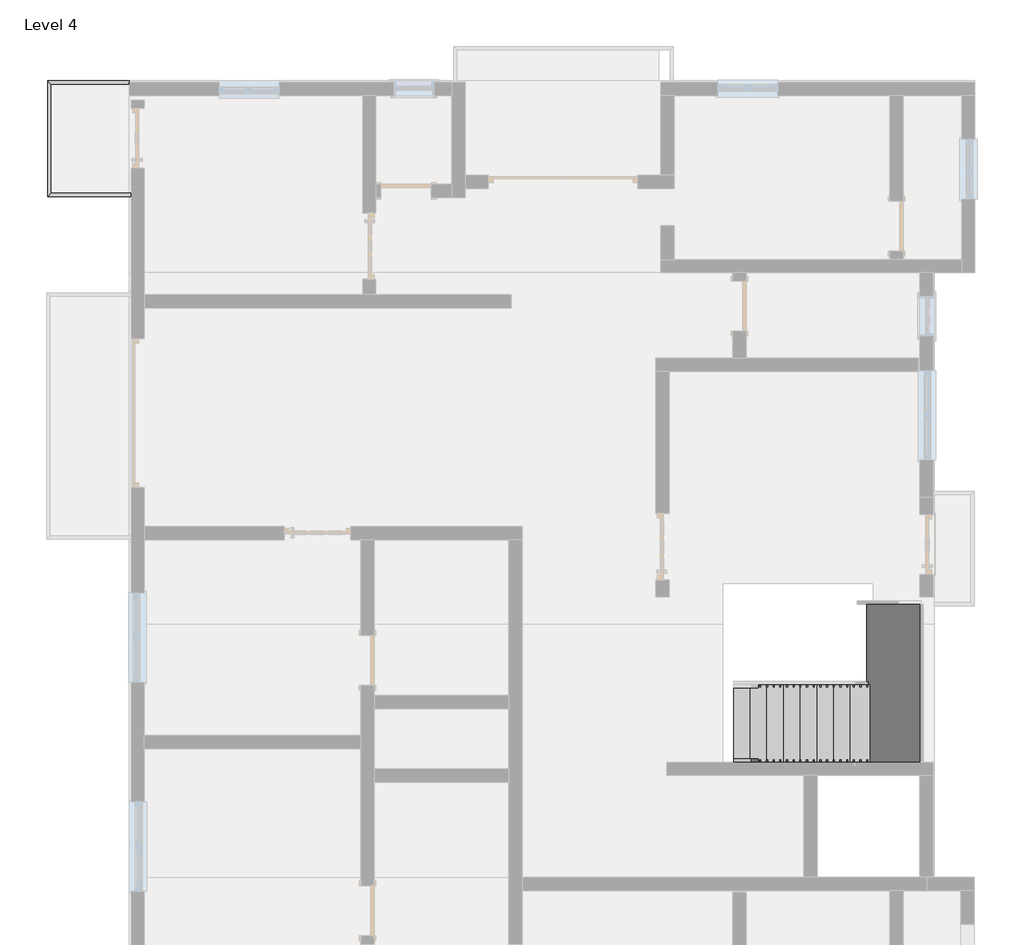
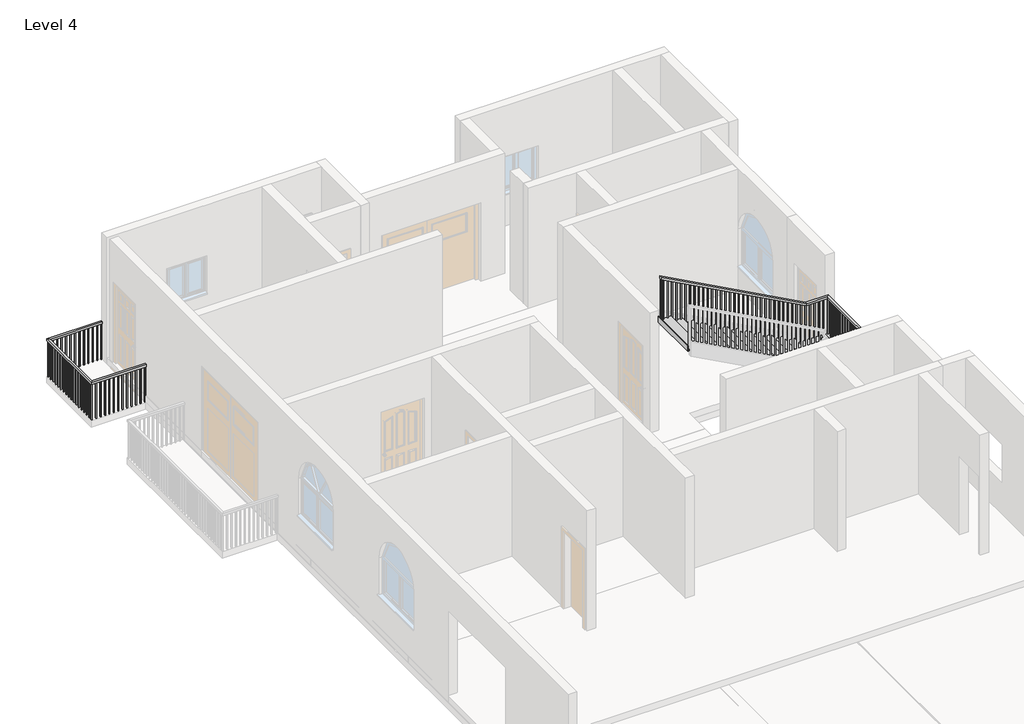
# One storey, part 5 of 7: 2 railings, 1 stair flight.
"""IFC4 building model written with IfcOpenShell, lengths in millimetres."""

from ifc_helpers import new_model, si_unit, frame, origin, place, context, project, spatial, polyline, outline, extrude, faceted_brep, transform, mapped, element, save
from components import stair_flight_9b376cb7

model = new_model("IFC4")

# Units and contexts
model_context = context("Model", 3, world=origin())
ifc_project = project(units=[si_unit("LENGTHUNIT", "METRE", prefix="MILLI")], contexts=[model_context])

# Site, building, storey
site = spatial("IfcSite", under=ifc_project)
building = spatial("IfcBuilding", under=site)
storey = spatial("IfcBuildingStorey", under=building, Name="Level 4", Elevation=9144.0)

# Railings
placement = place(None, origin())
element("IfcRailing", 1, ObjectType="Handrail - Rectangular", at=placement, inside=storey, context=model_context, shape_type="SolidModel", body=[
    faceted_brep([(-6354.2109037, 9376.4527313, 10058.4), (-6354.2109037, 9376.4527313, 10007.6), (-6354.2109037, 9427.2527313, 10007.6), (-6354.2109037, 9427.2527313, 10058.4), (-7548.0109037, 9376.4527313, 10058.4), (-7548.0109037, 9376.4527313, 10007.6), (-7598.8109037, 9427.2527313, 10007.6), (-7598.8109037, 9427.2527313, 10058.4), (-7548.0109037, 7717.9584215, 10058.4), (-7548.0109037, 7717.9584215, 10007.6), (-7598.8109037, 7667.1584215, 10007.6), (-7598.8109037, 7667.1584215, 10058.4), (-6330.8013636, 7717.9584215, 10058.4), (-6330.8013636, 7667.1584215, 10058.4), (-6330.8013636, 7667.1584215, 10007.6), (-6330.8013636, 7717.9584215, 10007.6)], [[[0, 1, 2, 3]], [[1, 0, 4, 5]], [[2, 1, 5, 6]], [[3, 2, 6, 7]], [[0, 3, 7, 4]], [[5, 4, 8, 9]], [[6, 5, 9, 10]], [[7, 6, 10, 11]], [[4, 7, 11, 8]], [[12, 13, 14, 15]], [[9, 8, 12, 15]], [[10, 9, 15, 14]], [[11, 10, 14, 13]], [[8, 11, 13, 12]]]),
    extrude(outline(polyline([(-6363.7359037, 7683.0334215), (-6363.7359037, 7702.0834215), (-6344.6859037, 7702.0834215), (-6344.6859037, 7683.0334215), (-6363.7359037, 7683.0334215)])), frame((0.0, 0.0, 9144.0), z_axis=(0.0, 0.0, 1.0), x_axis=(1.0, 0.0, 0.0)), (0.0, 0.0, 1.0), 863.6),
    extrude(outline(polyline([(-6465.3359037, 7683.0334215), (-6465.3359037, 7702.0834215), (-6446.2859037, 7702.0834215), (-6446.2859037, 7683.0334215), (-6465.3359037, 7683.0334215)])), frame((0.0, 0.0, 9144.0), z_axis=(0.0, 0.0, 1.0), x_axis=(1.0, 0.0, 0.0)), (0.0, 0.0, 1.0), 863.6),
    extrude(outline(polyline([(-6566.9359037, 7683.0334215), (-6566.9359037, 7702.0834215), (-6547.8859037, 7702.0834215), (-6547.8859037, 7683.0334215), (-6566.9359037, 7683.0334215)])), frame((0.0, 0.0, 9144.0), z_axis=(0.0, 0.0, 1.0), x_axis=(1.0, 0.0, 0.0)), (0.0, 0.0, 1.0), 863.6),
    extrude(outline(polyline([(-6668.5359037, 7683.0334215), (-6668.5359037, 7702.0834215), (-6649.4859037, 7702.0834215), (-6649.4859037, 7683.0334215), (-6668.5359037, 7683.0334215)])), frame((0.0, 0.0, 9144.0), z_axis=(0.0, 0.0, 1.0), x_axis=(1.0, 0.0, 0.0)), (0.0, 0.0, 1.0), 863.6),
    extrude(outline(polyline([(-6770.1359037, 7683.0334215), (-6770.1359037, 7702.0834215), (-6751.0859037, 7702.0834215), (-6751.0859037, 7683.0334215), (-6770.1359037, 7683.0334215)])), frame((0.0, 0.0, 9144.0), z_axis=(0.0, 0.0, 1.0), x_axis=(1.0, 0.0, 0.0)), (0.0, 0.0, 1.0), 863.6),
    extrude(outline(polyline([(-6871.7359037, 7683.0334215), (-6871.7359037, 7702.0834215), (-6852.6859037, 7702.0834215), (-6852.6859037, 7683.0334215), (-6871.7359037, 7683.0334215)])), frame((0.0, 0.0, 9144.0), z_axis=(0.0, 0.0, 1.0), x_axis=(1.0, 0.0, 0.0)), (0.0, 0.0, 1.0), 863.6),
    extrude(outline(polyline([(-6973.3359037, 7683.0334215), (-6973.3359037, 7702.0834215), (-6954.2859037, 7702.0834215), (-6954.2859037, 7683.0334215), (-6973.3359037, 7683.0334215)])), frame((0.0, 0.0, 9144.0), z_axis=(0.0, 0.0, 1.0), x_axis=(1.0, 0.0, 0.0)), (0.0, 0.0, 1.0), 863.6),
    extrude(outline(polyline([(-7074.9359037, 7683.0334215), (-7074.9359037, 7702.0834215), (-7055.8859037, 7702.0834215), (-7055.8859037, 7683.0334215), (-7074.9359037, 7683.0334215)])), frame((0.0, 0.0, 9144.0), z_axis=(0.0, 0.0, 1.0), x_axis=(1.0, 0.0, 0.0)), (0.0, 0.0, 1.0), 863.6),
    extrude(outline(polyline([(-7176.5359037, 7683.0334215), (-7176.5359037, 7702.0834215), (-7157.4859037, 7702.0834215), (-7157.4859037, 7683.0334215), (-7176.5359037, 7683.0334215)])), frame((0.0, 0.0, 9144.0), z_axis=(0.0, 0.0, 1.0), x_axis=(1.0, 0.0, 0.0)), (0.0, 0.0, 1.0), 863.6),
    extrude(outline(polyline([(-7278.1359037, 7683.0334215), (-7278.1359037, 7702.0834215), (-7259.0859037, 7702.0834215), (-7259.0859037, 7683.0334215), (-7278.1359037, 7683.0334215)])), frame((0.0, 0.0, 9144.0), z_axis=(0.0, 0.0, 1.0), x_axis=(1.0, 0.0, 0.0)), (0.0, 0.0, 1.0), 863.6),
    extrude(outline(polyline([(-7379.7359037, 7683.0334215), (-7379.7359037, 7702.0834215), (-7360.6859037, 7702.0834215), (-7360.6859037, 7683.0334215), (-7379.7359037, 7683.0334215)])), frame((0.0, 0.0, 9144.0), z_axis=(0.0, 0.0, 1.0), x_axis=(1.0, 0.0, 0.0)), (0.0, 0.0, 1.0), 863.6),
    extrude(outline(polyline([(-7481.3359037, 7683.0334215), (-7481.3359037, 7702.0834215), (-7462.2859037, 7702.0834215), (-7462.2859037, 7683.0334215), (-7481.3359037, 7683.0334215)])), frame((0.0, 0.0, 9144.0), z_axis=(0.0, 0.0, 1.0), x_axis=(1.0, 0.0, 0.0)), (0.0, 0.0, 1.0), 863.6),
    extrude(outline(polyline([(-7582.9359037, 7785.7777313), (-7563.8859037, 7785.7777313), (-7563.8859037, 7766.7277313), (-7582.9359037, 7766.7277313), (-7582.9359037, 7785.7777313)])), frame((0.0, 0.0, 9144.0), z_axis=(0.0, 0.0, 1.0), x_axis=(1.0, 0.0, 0.0)), (0.0, 0.0, 1.0), 863.6),
    extrude(outline(polyline([(-7582.9359037, 7887.3777313), (-7563.8859037, 7887.3777313), (-7563.8859037, 7868.3277313), (-7582.9359037, 7868.3277313), (-7582.9359037, 7887.3777313)])), frame((0.0, 0.0, 9144.0), z_axis=(0.0, 0.0, 1.0), x_axis=(1.0, 0.0, 0.0)), (0.0, 0.0, 1.0), 863.6),
    extrude(outline(polyline([(-7582.9359037, 7988.9777313), (-7563.8859037, 7988.9777313), (-7563.8859037, 7969.9277313), (-7582.9359037, 7969.9277313), (-7582.9359037, 7988.9777313)])), frame((0.0, 0.0, 9144.0), z_axis=(0.0, 0.0, 1.0), x_axis=(1.0, 0.0, 0.0)), (0.0, 0.0, 1.0), 863.6),
    extrude(outline(polyline([(-7582.9359037, 8090.5777313), (-7563.8859037, 8090.5777313), (-7563.8859037, 8071.5277313), (-7582.9359037, 8071.5277313), (-7582.9359037, 8090.5777313)])), frame((0.0, 0.0, 9144.0), z_axis=(0.0, 0.0, 1.0), x_axis=(1.0, 0.0, 0.0)), (0.0, 0.0, 1.0), 863.6),
    extrude(outline(polyline([(-7582.9359037, 8192.1777313), (-7563.8859037, 8192.1777313), (-7563.8859037, 8173.1277313), (-7582.9359037, 8173.1277313), (-7582.9359037, 8192.1777313)])), frame((0.0, 0.0, 9144.0), z_axis=(0.0, 0.0, 1.0), x_axis=(1.0, 0.0, 0.0)), (0.0, 0.0, 1.0), 863.6),
    extrude(outline(polyline([(-7582.9359037, 8293.7777313), (-7563.8859037, 8293.7777313), (-7563.8859037, 8274.7277313), (-7582.9359037, 8274.7277313), (-7582.9359037, 8293.7777313)])), frame((0.0, 0.0, 9144.0), z_axis=(0.0, 0.0, 1.0), x_axis=(1.0, 0.0, 0.0)), (0.0, 0.0, 1.0), 863.6),
    extrude(outline(polyline([(-7582.9359037, 8395.3777313), (-7563.8859037, 8395.3777313), (-7563.8859037, 8376.3277313), (-7582.9359037, 8376.3277313), (-7582.9359037, 8395.3777313)])), frame((0.0, 0.0, 9144.0), z_axis=(0.0, 0.0, 1.0), x_axis=(1.0, 0.0, 0.0)), (0.0, 0.0, 1.0), 863.6),
    extrude(outline(polyline([(-7582.9359037, 8496.9777313), (-7563.8859037, 8496.9777313), (-7563.8859037, 8477.9277313), (-7582.9359037, 8477.9277313), (-7582.9359037, 8496.9777313)])), frame((0.0, 0.0, 9144.0), z_axis=(0.0, 0.0, 1.0), x_axis=(1.0, 0.0, 0.0)), (0.0, 0.0, 1.0), 863.6),
    extrude(outline(polyline([(-7582.9359037, 8598.5777313), (-7563.8859037, 8598.5777313), (-7563.8859037, 8579.5277313), (-7582.9359037, 8579.5277313), (-7582.9359037, 8598.5777313)])), frame((0.0, 0.0, 9144.0), z_axis=(0.0, 0.0, 1.0), x_axis=(1.0, 0.0, 0.0)), (0.0, 0.0, 1.0), 863.6),
    extrude(outline(polyline([(-7582.9359037, 8700.1777313), (-7563.8859037, 8700.1777313), (-7563.8859037, 8681.1277313), (-7582.9359037, 8681.1277313), (-7582.9359037, 8700.1777313)])), frame((0.0, 0.0, 9144.0), z_axis=(0.0, 0.0, 1.0), x_axis=(1.0, 0.0, 0.0)), (0.0, 0.0, 1.0), 863.6),
    extrude(outline(polyline([(-7582.9359037, 8801.7777313), (-7563.8859037, 8801.7777313), (-7563.8859037, 8782.7277313), (-7582.9359037, 8782.7277313), (-7582.9359037, 8801.7777313)])), frame((0.0, 0.0, 9144.0), z_axis=(0.0, 0.0, 1.0), x_axis=(1.0, 0.0, 0.0)), (0.0, 0.0, 1.0), 863.6),
    extrude(outline(polyline([(-7582.9359037, 8903.3777313), (-7563.8859037, 8903.3777313), (-7563.8859037, 8884.3277313), (-7582.9359037, 8884.3277313), (-7582.9359037, 8903.3777313)])), frame((0.0, 0.0, 9144.0), z_axis=(0.0, 0.0, 1.0), x_axis=(1.0, 0.0, 0.0)), (0.0, 0.0, 1.0), 863.6),
    extrude(outline(polyline([(-7582.9359037, 9004.9777313), (-7563.8859037, 9004.9777313), (-7563.8859037, 8985.9277313), (-7582.9359037, 8985.9277313), (-7582.9359037, 9004.9777313)])), frame((0.0, 0.0, 9144.0), z_axis=(0.0, 0.0, 1.0), x_axis=(1.0, 0.0, 0.0)), (0.0, 0.0, 1.0), 863.6),
    extrude(outline(polyline([(-7582.9359037, 9106.5777313), (-7563.8859037, 9106.5777313), (-7563.8859037, 9087.5277313), (-7582.9359037, 9087.5277313), (-7582.9359037, 9106.5777313)])), frame((0.0, 0.0, 9144.0), z_axis=(0.0, 0.0, 1.0), x_axis=(1.0, 0.0, 0.0)), (0.0, 0.0, 1.0), 863.6),
    extrude(outline(polyline([(-7582.9359037, 9208.1777313), (-7563.8859037, 9208.1777313), (-7563.8859037, 9189.1277313), (-7582.9359037, 9189.1277313), (-7582.9359037, 9208.1777313)])), frame((0.0, 0.0, 9144.0), z_axis=(0.0, 0.0, 1.0), x_axis=(1.0, 0.0, 0.0)), (0.0, 0.0, 1.0), 863.6),
    extrude(outline(polyline([(-7582.9359037, 9309.7777313), (-7563.8859037, 9309.7777313), (-7563.8859037, 9290.7277313), (-7582.9359037, 9290.7277313), (-7582.9359037, 9309.7777313)])), frame((0.0, 0.0, 9144.0), z_axis=(0.0, 0.0, 1.0), x_axis=(1.0, 0.0, 0.0)), (0.0, 0.0, 1.0), 863.6),
    extrude(outline(polyline([(-7462.2859037, 9411.3777313), (-7462.2859037, 9392.3277313), (-7481.3359037, 9392.3277313), (-7481.3359037, 9411.3777313), (-7462.2859037, 9411.3777313)])), frame((0.0, 0.0, 9144.0), z_axis=(0.0, 0.0, 1.0), x_axis=(1.0, 0.0, 0.0)), (0.0, 0.0, 1.0), 863.6),
    extrude(outline(polyline([(-7360.6859037, 9411.3777313), (-7360.6859037, 9392.3277313), (-7379.7359037, 9392.3277313), (-7379.7359037, 9411.3777313), (-7360.6859037, 9411.3777313)])), frame((0.0, 0.0, 9144.0), z_axis=(0.0, 0.0, 1.0), x_axis=(1.0, 0.0, 0.0)), (0.0, 0.0, 1.0), 863.6),
    extrude(outline(polyline([(-7259.0859037, 9411.3777313), (-7259.0859037, 9392.3277313), (-7278.1359037, 9392.3277313), (-7278.1359037, 9411.3777313), (-7259.0859037, 9411.3777313)])), frame((0.0, 0.0, 9144.0), z_axis=(0.0, 0.0, 1.0), x_axis=(1.0, 0.0, 0.0)), (0.0, 0.0, 1.0), 863.6),
    extrude(outline(polyline([(-7157.4859037, 9411.3777313), (-7157.4859037, 9392.3277313), (-7176.5359037, 9392.3277313), (-7176.5359037, 9411.3777313), (-7157.4859037, 9411.3777313)])), frame((0.0, 0.0, 9144.0), z_axis=(0.0, 0.0, 1.0), x_axis=(1.0, 0.0, 0.0)), (0.0, 0.0, 1.0), 863.6),
    extrude(outline(polyline([(-7055.8859037, 9411.3777313), (-7055.8859037, 9392.3277313), (-7074.9359037, 9392.3277313), (-7074.9359037, 9411.3777313), (-7055.8859037, 9411.3777313)])), frame((0.0, 0.0, 9144.0), z_axis=(0.0, 0.0, 1.0), x_axis=(1.0, 0.0, 0.0)), (0.0, 0.0, 1.0), 863.6),
    extrude(outline(polyline([(-6954.2859037, 9411.3777313), (-6954.2859037, 9392.3277313), (-6973.3359037, 9392.3277313), (-6973.3359037, 9411.3777313), (-6954.2859037, 9411.3777313)])), frame((0.0, 0.0, 9144.0), z_axis=(0.0, 0.0, 1.0), x_axis=(1.0, 0.0, 0.0)), (0.0, 0.0, 1.0), 863.6),
    extrude(outline(polyline([(-6852.6859037, 9411.3777313), (-6852.6859037, 9392.3277313), (-6871.7359037, 9392.3277313), (-6871.7359037, 9411.3777313), (-6852.6859037, 9411.3777313)])), frame((0.0, 0.0, 9144.0), z_axis=(0.0, 0.0, 1.0), x_axis=(1.0, 0.0, 0.0)), (0.0, 0.0, 1.0), 863.6),
    extrude(outline(polyline([(-6751.0859037, 9411.3777313), (-6751.0859037, 9392.3277313), (-6770.1359037, 9392.3277313), (-6770.1359037, 9411.3777313), (-6751.0859037, 9411.3777313)])), frame((0.0, 0.0, 9144.0), z_axis=(0.0, 0.0, 1.0), x_axis=(1.0, 0.0, 0.0)), (0.0, 0.0, 1.0), 863.6),
    extrude(outline(polyline([(-6649.4859037, 9411.3777313), (-6649.4859037, 9392.3277313), (-6668.5359037, 9392.3277313), (-6668.5359037, 9411.3777313), (-6649.4859037, 9411.3777313)])), frame((0.0, 0.0, 9144.0), z_axis=(0.0, 0.0, 1.0), x_axis=(1.0, 0.0, 0.0)), (0.0, 0.0, 1.0), 863.6),
    extrude(outline(polyline([(-6547.8859037, 9411.3777313), (-6547.8859037, 9392.3277313), (-6566.9359037, 9392.3277313), (-6566.9359037, 9411.3777313), (-6547.8859037, 9411.3777313)])), frame((0.0, 0.0, 9144.0), z_axis=(0.0, 0.0, 1.0), x_axis=(1.0, 0.0, 0.0)), (0.0, 0.0, 1.0), 863.6),
    extrude(outline(polyline([(-6446.2859037, 9411.3777313), (-6446.2859037, 9392.3277313), (-6465.3359037, 9392.3277313), (-6465.3359037, 9411.3777313), (-6446.2859037, 9411.3777313)])), frame((0.0, 0.0, 9144.0), z_axis=(0.0, 0.0, 1.0), x_axis=(1.0, 0.0, 0.0)), (0.0, 0.0, 1.0), 863.6),
    extrude(outline(polyline([(-7582.9359037, 7702.0834215), (-7563.8859037, 7702.0834215), (-7563.8859037, 7683.0334215), (-7582.9359037, 7683.0334215), (-7582.9359037, 7702.0834215)])), frame((0.0, 0.0, 9144.0), z_axis=(0.0, 0.0, 1.0), x_axis=(1.0, 0.0, 0.0)), (0.0, 0.0, 1.0), 863.6),
    extrude(outline(polyline([(-7563.8859037, 9411.3777313), (-7563.8859037, 9392.3277313), (-7582.9359037, 9392.3277313), (-7582.9359037, 9411.3777313), (-7563.8859037, 9411.3777313)])), frame((0.0, 0.0, 9144.0), z_axis=(0.0, 0.0, 1.0), x_axis=(1.0, 0.0, 0.0)), (0.0, 0.0, 1.0), 863.6),
    extrude(outline(polyline([(-6349.8513636, 7683.0334215), (-6349.8513636, 7702.0834215), (-6330.8013636, 7702.0834215), (-6330.8013636, 7683.0334215), (-6349.8513636, 7683.0334215)])), frame((0.0, 0.0, 9144.0), z_axis=(0.0, 0.0, 1.0), x_axis=(1.0, 0.0, 0.0)), (0.0, 0.0, 1.0), 863.6),
    extrude(outline(polyline([(-6354.2109037, 9411.3777313), (-6354.2109037, 9392.3277313), (-6373.2609037, 9392.3277313), (-6373.2609037, 9411.3777313), (-6354.2109037, 9411.3777313)])), frame((0.0, 0.0, 9144.0), z_axis=(0.0, 0.0, 1.0), x_axis=(1.0, 0.0, 0.0)), (0.0, 0.0, 1.0), 863.6),
])
element("IfcRailing", 2, ObjectType="Handrail - Rectangular", at=placement, inside=storey, context=model_context, shape_type="SolidModel", body=[
    faceted_brep([(2827.8890963, -884.7037749, 10196.9454545), (2827.8890963, -884.7037749, 10139.2159002), (2827.8890963, -935.5037749, 10139.2159002), (2827.8890963, -935.5037749, 10196.9454545), (4881.0326586, -884.7037749, 11305.3090909), (4893.8690324, -884.7037749, 11254.5090909), (4893.8690324, -935.5037749, 11254.5090909), (4881.0326586, -935.5037749, 11305.3090909), (5609.1890963, 1413.9962251, 11254.5090909), (5609.1890963, 1413.9962251, 11305.3090909), (5136.7946221, 1413.9962251, 11305.3090909), (5123.9193635, 1413.9962251, 11254.5090909), (5659.9890963, 1464.7962251, 11254.5090909), (5123.9193635, 1464.7962251, 11254.5090909), (5659.9890963, 1464.7962251, 11305.3090909), (5136.7946221, 1464.7962251, 11305.3090909), (5609.1890963, -884.7037749, 11305.3090909), (5609.1890963, -884.7037749, 11254.5090909), (5659.9890963, -935.5037749, 11254.5090909), (5659.9890963, -935.5037749, 11305.3090909), (1811.8890963, 1413.9962251, 13106.4), (1811.8890963, 1464.7962251, 13106.4), (1811.8890963, 1464.7962251, 13048.6255127), (1811.8890963, 1413.9962251, 13048.6255127)], [[[0, 1, 2, 3]], [[1, 0, 4, 5]], [[2, 1, 5, 6]], [[3, 2, 6, 7]], [[0, 3, 7, 4]], [[8, 9, 10, 11]], [[12, 8, 11, 13]], [[14, 12, 13, 15]], [[9, 14, 15, 10]], [[5, 4, 16, 17]], [[6, 5, 17, 18]], [[7, 6, 18, 19]], [[4, 7, 19, 16]], [[17, 16, 9, 8]], [[18, 17, 8, 12]], [[19, 18, 12, 14]], [[16, 19, 14, 9]], [[20, 21, 22, 23]], [[11, 10, 20, 23]], [[13, 11, 23, 22]], [[15, 13, 22, 21]], [[10, 15, 21, 20]]]),
    extrude(outline(polyline([(13008.9709526, 1884.9140963), (13019.2548546, 1865.8640963), (12053.4545455, 1865.8640963), (12053.4545455, 1884.9140963), (13008.9709526, 1884.9140963)])), frame((0.0, 1429.8712251, 0.0), z_axis=(0.0, 1.0, 0.0), x_axis=(0.0, 0.0, 1.0)), (0.0, 0.0, 1.0), 19.05),
    extrude(outline(polyline([(12954.0316972, 1986.5140963), (12964.3510225, 1967.4640963), (12053.4545455, 1967.4640963), (12053.4545455, 1986.5140963), (12954.0316972, 1986.5140963)])), frame((0.0, 1429.8712251, 0.0), z_axis=(0.0, 1.0, 0.0), x_axis=(0.0, 0.0, 1.0)), (0.0, 0.0, 1.0), 19.05),
    extrude(outline(polyline([(12898.9952954, 2088.1140963), (12909.3146207, 2069.0640963), (11914.9090909, 2069.0640963), (11914.9090909, 2088.1140963), (12898.9952954, 2088.1140963)])), frame((0.0, 1429.8712251, 0.0), z_axis=(0.0, 1.0, 0.0), x_axis=(0.0, 0.0, 1.0)), (0.0, 0.0, 1.0), 19.05),
    extrude(outline(polyline([(12843.9588936, 2189.7140963), (12854.278219, 2170.6640963), (11914.9090909, 2170.6640963), (11914.9090909, 2189.7140963), (12843.9588936, 2189.7140963)])), frame((0.0, 1429.8712251, 0.0), z_axis=(0.0, 1.0, 0.0), x_axis=(0.0, 0.0, 1.0)), (0.0, 0.0, 1.0), 19.05),
    extrude(outline(polyline([(12788.9224919, 2291.3140963), (12799.2418172, 2272.2640963), (11914.9090909, 2272.2640963), (11914.9090909, 2291.3140963), (12788.9224919, 2291.3140963)])), frame((0.0, 1429.8712251, 0.0), z_axis=(0.0, 1.0, 0.0), x_axis=(0.0, 0.0, 1.0)), (0.0, 0.0, 1.0), 19.05),
    extrude(outline(polyline([(12733.8860901, 2392.9140963), (12744.2054154, 2373.8640963), (11776.3636364, 2373.8640963), (11776.3636364, 2392.9140963), (12733.8860901, 2392.9140963)])), frame((0.0, 1429.8712251, 0.0), z_axis=(0.0, 1.0, 0.0), x_axis=(0.0, 0.0, 1.0)), (0.0, 0.0, 1.0), 19.05),
    extrude(outline(polyline([(12678.8496883, 2494.5140963), (12689.1690137, 2475.4640963), (11776.3636364, 2475.4640963), (11776.3636364, 2494.5140963), (12678.8496883, 2494.5140963)])), frame((0.0, 1429.8712251, 0.0), z_axis=(0.0, 1.0, 0.0), x_axis=(0.0, 0.0, 1.0)), (0.0, 0.0, 1.0), 19.05),
    extrude(outline(polyline([(12623.8132866, 2596.1140963), (12634.1326119, 2577.0640963), (11637.8181818, 2577.0640963), (11637.8181818, 2596.1140963), (12623.8132866, 2596.1140963)])), frame((0.0, 1429.8712251, 0.0), z_axis=(0.0, 1.0, 0.0), x_axis=(0.0, 0.0, 1.0)), (0.0, 0.0, 1.0), 19.05),
    extrude(outline(polyline([(12568.7768848, 2697.7140963), (12579.0962101, 2678.6640963), (11637.8181818, 2678.6640963), (11637.8181818, 2697.7140963), (12568.7768848, 2697.7140963)])), frame((0.0, 1429.8712251, 0.0), z_axis=(0.0, 1.0, 0.0), x_axis=(0.0, 0.0, 1.0)), (0.0, 0.0, 1.0), 19.05),
    extrude(outline(polyline([(12513.740483, 2799.3140963), (12524.0598084, 2780.2640963), (11637.8181818, 2780.2640963), (11637.8181818, 2799.3140963), (12513.740483, 2799.3140963)])), frame((0.0, 1429.8712251, 0.0), z_axis=(0.0, 1.0, 0.0), x_axis=(0.0, 0.0, 1.0)), (0.0, 0.0, 1.0), 19.05),
    extrude(outline(polyline([(12458.7040813, 2900.9140963), (12469.0234066, 2881.8640963), (11499.2727273, 2881.8640963), (11499.2727273, 2900.9140963), (12458.7040813, 2900.9140963)])), frame((0.0, 1429.8712251, 0.0), z_axis=(0.0, 1.0, 0.0), x_axis=(0.0, 0.0, 1.0)), (0.0, 0.0, 1.0), 19.05),
    extrude(outline(polyline([(12403.6676795, 3002.5140963), (12413.9870048, 2983.4640963), (11499.2727273, 2983.4640963), (11499.2727273, 3002.5140963), (12403.6676795, 3002.5140963)])), frame((0.0, 1429.8712251, 0.0), z_axis=(0.0, 1.0, 0.0), x_axis=(0.0, 0.0, 1.0)), (0.0, 0.0, 1.0), 19.05),
    extrude(outline(polyline([(12348.6312777, 3104.1140963), (12358.9506031, 3085.0640963), (11360.7272727, 3085.0640963), (11360.7272727, 3104.1140963), (12348.6312777, 3104.1140963)])), frame((0.0, 1429.8712251, 0.0), z_axis=(0.0, 1.0, 0.0), x_axis=(0.0, 0.0, 1.0)), (0.0, 0.0, 1.0), 19.05),
    extrude(outline(polyline([(12293.594876, 3205.7140963), (12303.9142013, 3186.6640963), (11360.7272727, 3186.6640963), (11360.7272727, 3205.7140963), (12293.594876, 3205.7140963)])), frame((0.0, 1429.8712251, 0.0), z_axis=(0.0, 1.0, 0.0), x_axis=(0.0, 0.0, 1.0)), (0.0, 0.0, 1.0), 19.05),
    extrude(outline(polyline([(12238.5584742, 3307.3140963), (12248.8777995, 3288.2640963), (11360.7272727, 3288.2640963), (11360.7272727, 3307.3140963), (12238.5584742, 3307.3140963)])), frame((0.0, 1429.8712251, 0.0), z_axis=(0.0, 1.0, 0.0), x_axis=(0.0, 0.0, 1.0)), (0.0, 0.0, 1.0), 19.05),
    extrude(outline(polyline([(12183.4052679, 3408.9140963), (12193.6891699, 3389.8640963), (11222.1818182, 3389.8640963), (11222.1818182, 3408.9140963), (12183.4052679, 3408.9140963)])), frame((0.0, 1429.8712251, 0.0), z_axis=(0.0, 1.0, 0.0), x_axis=(0.0, 0.0, 1.0)), (0.0, 0.0, 1.0), 19.05),
    extrude(outline(polyline([(12128.4856707, 3510.5140963), (12138.804996, 3491.4640963), (11222.1818182, 3491.4640963), (11222.1818182, 3510.5140963), (12128.4856707, 3510.5140963)])), frame((0.0, 1429.8712251, 0.0), z_axis=(0.0, 1.0, 0.0), x_axis=(0.0, 0.0, 1.0)), (0.0, 0.0, 1.0), 19.05),
    extrude(outline(polyline([(12073.4492689, 3612.1140963), (12083.7685942, 3593.0640963), (11083.6363636, 3593.0640963), (11083.6363636, 3612.1140963), (12073.4492689, 3612.1140963)])), frame((0.0, 1429.8712251, 0.0), z_axis=(0.0, 1.0, 0.0), x_axis=(0.0, 0.0, 1.0)), (0.0, 0.0, 1.0), 19.05),
    extrude(outline(polyline([(12018.4128671, 3713.7140963), (12028.7321924, 3694.6640963), (11083.6363636, 3694.6640963), (11083.6363636, 3713.7140963), (12018.4128671, 3713.7140963)])), frame((0.0, 1429.8712251, 0.0), z_axis=(0.0, 1.0, 0.0), x_axis=(0.0, 0.0, 1.0)), (0.0, 0.0, 1.0), 19.05),
    extrude(outline(polyline([(11963.3764653, 3815.3140963), (11973.6957907, 3796.2640963), (11083.6363636, 3796.2640963), (11083.6363636, 3815.3140963), (11963.3764653, 3815.3140963)])), frame((0.0, 1429.8712251, 0.0), z_axis=(0.0, 1.0, 0.0), x_axis=(0.0, 0.0, 1.0)), (0.0, 0.0, 1.0), 19.05),
    extrude(outline(polyline([(11908.3400636, 3916.9140963), (11918.6593889, 3897.8640963), (10945.0909091, 3897.8640963), (10945.0909091, 3916.9140963), (11908.3400636, 3916.9140963)])), frame((0.0, 1429.8712251, 0.0), z_axis=(0.0, 1.0, 0.0), x_axis=(0.0, 0.0, 1.0)), (0.0, 0.0, 1.0), 19.05),
    extrude(outline(polyline([(11853.3036618, 4018.5140963), (11863.6229871, 3999.4640963), (10945.0909091, 3999.4640963), (10945.0909091, 4018.5140963), (11853.3036618, 4018.5140963)])), frame((0.0, 1429.8712251, 0.0), z_axis=(0.0, 1.0, 0.0), x_axis=(0.0, 0.0, 1.0)), (0.0, 0.0, 1.0), 19.05),
    extrude(outline(polyline([(11798.26726, 4120.1140963), (11808.5865854, 4101.0640963), (10806.5454545, 4101.0640963), (10806.5454545, 4120.1140963), (11798.26726, 4120.1140963)])), frame((0.0, 1429.8712251, 0.0), z_axis=(0.0, 1.0, 0.0), x_axis=(0.0, 0.0, 1.0)), (0.0, 0.0, 1.0), 19.05),
    extrude(outline(polyline([(11743.2308583, 4221.7140963), (11753.5501836, 4202.6640963), (10806.5454545, 4202.6640963), (10806.5454545, 4221.7140963), (11743.2308583, 4221.7140963)])), frame((0.0, 1429.8712251, 0.0), z_axis=(0.0, 1.0, 0.0), x_axis=(0.0, 0.0, 1.0)), (0.0, 0.0, 1.0), 19.05),
    extrude(outline(polyline([(11688.1944565, 4323.3140963), (11698.5137818, 4304.2640963), (10806.5454545, 4304.2640963), (10806.5454545, 4323.3140963), (11688.1944565, 4323.3140963)])), frame((0.0, 1429.8712251, 0.0), z_axis=(0.0, 1.0, 0.0), x_axis=(0.0, 0.0, 1.0)), (0.0, 0.0, 1.0), 19.05),
    extrude(outline(polyline([(11633.1580547, 4424.9140963), (11643.4773801, 4405.8640963), (10668.0, 4405.8640963), (10668.0, 4424.9140963), (11633.1580547, 4424.9140963)])), frame((0.0, 1429.8712251, 0.0), z_axis=(0.0, 1.0, 0.0), x_axis=(0.0, 0.0, 1.0)), (0.0, 0.0, 1.0), 19.05),
    extrude(outline(polyline([(11578.100517, 4526.5140963), (11588.384419, 4507.4640963), (10668.0, 4507.4640963), (10668.0, 4526.5140963), (11578.100517, 4526.5140963)])), frame((0.0, 1429.8712251, 0.0), z_axis=(0.0, 1.0, 0.0), x_axis=(0.0, 0.0, 1.0)), (0.0, 0.0, 1.0), 19.05),
    extrude(outline(polyline([(11523.0852512, 4628.1140963), (11533.4045765, 4609.0640963), (10529.4545455, 4609.0640963), (10529.4545455, 4628.1140963), (11523.0852512, 4628.1140963)])), frame((0.0, 1429.8712251, 0.0), z_axis=(0.0, 1.0, 0.0), x_axis=(0.0, 0.0, 1.0)), (0.0, 0.0, 1.0), 19.05),
    extrude(outline(polyline([(11468.0488494, 4729.7140963), (11478.3681748, 4710.6640963), (10529.4545455, 4710.6640963), (10529.4545455, 4729.7140963), (11468.0488494, 4729.7140963)])), frame((0.0, 1429.8712251, 0.0), z_axis=(0.0, 1.0, 0.0), x_axis=(0.0, 0.0, 1.0)), (0.0, 0.0, 1.0), 19.05),
    extrude(outline(polyline([(11413.0124477, 4831.3140963), (11423.331773, 4812.2640963), (10529.4545455, 4812.2640963), (10529.4545455, 4831.3140963), (11413.0124477, 4831.3140963)])), frame((0.0, 1429.8712251, 0.0), z_axis=(0.0, 1.0, 0.0), x_axis=(0.0, 0.0, 1.0)), (0.0, 0.0, 1.0), 19.05),
    extrude(outline(polyline([(11357.9760459, 4932.9140963), (11368.2953712, 4913.8640963), (10390.9090909, 4913.8640963), (10390.9090909, 4932.9140963), (11357.9760459, 4932.9140963)])), frame((0.0, 1429.8712251, 0.0), z_axis=(0.0, 1.0, 0.0), x_axis=(0.0, 0.0, 1.0)), (0.0, 0.0, 1.0), 19.05),
    extrude(outline(polyline([(11302.9396441, 5034.5140963), (11313.2589695, 5015.4640963), (10390.9090909, 5015.4640963), (10390.9090909, 5034.5140963), (11302.9396441, 5034.5140963)])), frame((0.0, 1429.8712251, 0.0), z_axis=(0.0, 1.0, 0.0), x_axis=(0.0, 0.0, 1.0)), (0.0, 0.0, 1.0), 19.05),
    extrude(outline(polyline([(11247.9032424, 5136.1140963), (11258.2225677, 5117.0640963), (10390.9090909, 5117.0640963), (10390.9090909, 5136.1140963), (11247.9032424, 5136.1140963)])), frame((0.0, 1429.8712251, 0.0), z_axis=(0.0, 1.0, 0.0), x_axis=(0.0, 0.0, 1.0)), (0.0, 0.0, 1.0), 19.05),
    extrude(outline(polyline([(5237.7140963, 1448.9212251), (5237.7140963, 1429.8712251), (5218.6640963, 1429.8712251), (5218.6640963, 1448.9212251), (5237.7140963, 1448.9212251)])), frame((0.0, 0.0, 10390.9090909), z_axis=(0.0, 0.0, 1.0), x_axis=(1.0, 0.0, 0.0)), (0.0, 0.0, 1.0), 863.6),
    extrude(outline(polyline([(5339.3140963, 1448.9212251), (5339.3140963, 1429.8712251), (5320.2640963, 1429.8712251), (5320.2640963, 1448.9212251), (5339.3140963, 1448.9212251)])), frame((0.0, 0.0, 10390.9090909), z_axis=(0.0, 0.0, 1.0), x_axis=(1.0, 0.0, 0.0)), (0.0, 0.0, 1.0), 863.6),
    extrude(outline(polyline([(5440.9140963, 1448.9212251), (5440.9140963, 1429.8712251), (5421.8640963, 1429.8712251), (5421.8640963, 1448.9212251), (5440.9140963, 1448.9212251)])), frame((0.0, 0.0, 10390.9090909), z_axis=(0.0, 0.0, 1.0), x_axis=(1.0, 0.0, 0.0)), (0.0, 0.0, 1.0), 863.6),
    extrude(outline(polyline([(5542.5140963, 1448.9212251), (5542.5140963, 1429.8712251), (5523.4640963, 1429.8712251), (5523.4640963, 1448.9212251), (5542.5140963, 1448.9212251)])), frame((0.0, 0.0, 10390.9090909), z_axis=(0.0, 0.0, 1.0), x_axis=(1.0, 0.0, 0.0)), (0.0, 0.0, 1.0), 863.6),
    extrude(outline(polyline([(5644.1140963, 1417.1712251), (5625.0640963, 1417.1712251), (5625.0640963, 1436.2212251), (5644.1140963, 1436.2212251), (5644.1140963, 1417.1712251)])), frame((0.0, 0.0, 10390.9090909), z_axis=(0.0, 0.0, 1.0), x_axis=(1.0, 0.0, 0.0)), (0.0, 0.0, 1.0), 863.6),
    extrude(outline(polyline([(5644.1140963, 1315.5712251), (5625.0640963, 1315.5712251), (5625.0640963, 1334.6212251), (5644.1140963, 1334.6212251), (5644.1140963, 1315.5712251)])), frame((0.0, 0.0, 10390.9090909), z_axis=(0.0, 0.0, 1.0), x_axis=(1.0, 0.0, 0.0)), (0.0, 0.0, 1.0), 863.6),
    extrude(outline(polyline([(5644.1140963, 1213.9712251), (5625.0640963, 1213.9712251), (5625.0640963, 1233.0212251), (5644.1140963, 1233.0212251), (5644.1140963, 1213.9712251)])), frame((0.0, 0.0, 10390.9090909), z_axis=(0.0, 0.0, 1.0), x_axis=(1.0, 0.0, 0.0)), (0.0, 0.0, 1.0), 863.6),
    extrude(outline(polyline([(5644.1140963, 1112.3712251), (5625.0640963, 1112.3712251), (5625.0640963, 1131.4212251), (5644.1140963, 1131.4212251), (5644.1140963, 1112.3712251)])), frame((0.0, 0.0, 10390.9090909), z_axis=(0.0, 0.0, 1.0), x_axis=(1.0, 0.0, 0.0)), (0.0, 0.0, 1.0), 863.6),
    extrude(outline(polyline([(5644.1140963, 1010.7712251), (5625.0640963, 1010.7712251), (5625.0640963, 1029.8212251), (5644.1140963, 1029.8212251), (5644.1140963, 1010.7712251)])), frame((0.0, 0.0, 10390.9090909), z_axis=(0.0, 0.0, 1.0), x_axis=(1.0, 0.0, 0.0)), (0.0, 0.0, 1.0), 863.6),
    extrude(outline(polyline([(5644.1140963, 909.1712251), (5625.0640963, 909.1712251), (5625.0640963, 928.2212251), (5644.1140963, 928.2212251), (5644.1140963, 909.1712251)])), frame((0.0, 0.0, 10390.9090909), z_axis=(0.0, 0.0, 1.0), x_axis=(1.0, 0.0, 0.0)), (0.0, 0.0, 1.0), 863.6),
    extrude(outline(polyline([(5644.1140963, 807.5712251), (5625.0640963, 807.5712251), (5625.0640963, 826.6212251), (5644.1140963, 826.6212251), (5644.1140963, 807.5712251)])), frame((0.0, 0.0, 10390.9090909), z_axis=(0.0, 0.0, 1.0), x_axis=(1.0, 0.0, 0.0)), (0.0, 0.0, 1.0), 863.6),
    extrude(outline(polyline([(5644.1140963, 705.9712251), (5625.0640963, 705.9712251), (5625.0640963, 725.0212251), (5644.1140963, 725.0212251), (5644.1140963, 705.9712251)])), frame((0.0, 0.0, 10390.9090909), z_axis=(0.0, 0.0, 1.0), x_axis=(1.0, 0.0, 0.0)), (0.0, 0.0, 1.0), 863.6),
    extrude(outline(polyline([(5644.1140963, 604.3712251), (5625.0640963, 604.3712251), (5625.0640963, 623.4212251), (5644.1140963, 623.4212251), (5644.1140963, 604.3712251)])), frame((0.0, 0.0, 10390.9090909), z_axis=(0.0, 0.0, 1.0), x_axis=(1.0, 0.0, 0.0)), (0.0, 0.0, 1.0), 863.6),
    extrude(outline(polyline([(5644.1140963, 502.7712251), (5625.0640963, 502.7712251), (5625.0640963, 521.8212251), (5644.1140963, 521.8212251), (5644.1140963, 502.7712251)])), frame((0.0, 0.0, 10390.9090909), z_axis=(0.0, 0.0, 1.0), x_axis=(1.0, 0.0, 0.0)), (0.0, 0.0, 1.0), 863.6),
    extrude(outline(polyline([(5644.1140963, 401.1712251), (5625.0640963, 401.1712251), (5625.0640963, 420.2212251), (5644.1140963, 420.2212251), (5644.1140963, 401.1712251)])), frame((0.0, 0.0, 10390.9090909), z_axis=(0.0, 0.0, 1.0), x_axis=(1.0, 0.0, 0.0)), (0.0, 0.0, 1.0), 863.6),
    extrude(outline(polyline([(5644.1140963, 299.5712251), (5625.0640963, 299.5712251), (5625.0640963, 318.6212251), (5644.1140963, 318.6212251), (5644.1140963, 299.5712251)])), frame((0.0, 0.0, 10390.9090909), z_axis=(0.0, 0.0, 1.0), x_axis=(1.0, 0.0, 0.0)), (0.0, 0.0, 1.0), 863.6),
    extrude(outline(polyline([(5644.1140963, 197.9712251), (5625.0640963, 197.9712251), (5625.0640963, 217.0212251), (5644.1140963, 217.0212251), (5644.1140963, 197.9712251)])), frame((0.0, 0.0, 10390.9090909), z_axis=(0.0, 0.0, 1.0), x_axis=(1.0, 0.0, 0.0)), (0.0, 0.0, 1.0), 863.6),
    extrude(outline(polyline([(5644.1140963, 96.3712251), (5625.0640963, 96.3712251), (5625.0640963, 115.4212251), (5644.1140963, 115.4212251), (5644.1140963, 96.3712251)])), frame((0.0, 0.0, 10390.9090909), z_axis=(0.0, 0.0, 1.0), x_axis=(1.0, 0.0, 0.0)), (0.0, 0.0, 1.0), 863.6),
    extrude(outline(polyline([(5644.1140963, -5.2287749), (5625.0640963, -5.2287749), (5625.0640963, 13.8212251), (5644.1140963, 13.8212251), (5644.1140963, -5.2287749)])), frame((0.0, 0.0, 10390.9090909), z_axis=(0.0, 0.0, 1.0), x_axis=(1.0, 0.0, 0.0)), (0.0, 0.0, 1.0), 863.6),
    extrude(outline(polyline([(5644.1140963, -106.8287749), (5625.0640963, -106.8287749), (5625.0640963, -87.7787749), (5644.1140963, -87.7787749), (5644.1140963, -106.8287749)])), frame((0.0, 0.0, 10390.9090909), z_axis=(0.0, 0.0, 1.0), x_axis=(1.0, 0.0, 0.0)), (0.0, 0.0, 1.0), 863.6),
    extrude(outline(polyline([(5644.1140963, -208.4287749), (5625.0640963, -208.4287749), (5625.0640963, -189.3787749), (5644.1140963, -189.3787749), (5644.1140963, -208.4287749)])), frame((0.0, 0.0, 10390.9090909), z_axis=(0.0, 0.0, 1.0), x_axis=(1.0, 0.0, 0.0)), (0.0, 0.0, 1.0), 863.6),
    extrude(outline(polyline([(5644.1140963, -310.0287749), (5625.0640963, -310.0287749), (5625.0640963, -290.9787749), (5644.1140963, -290.9787749), (5644.1140963, -310.0287749)])), frame((0.0, 0.0, 10390.9090909), z_axis=(0.0, 0.0, 1.0), x_axis=(1.0, 0.0, 0.0)), (0.0, 0.0, 1.0), 863.6),
    extrude(outline(polyline([(5644.1140963, -411.6287749), (5625.0640963, -411.6287749), (5625.0640963, -392.5787749), (5644.1140963, -392.5787749), (5644.1140963, -411.6287749)])), frame((0.0, 0.0, 10390.9090909), z_axis=(0.0, 0.0, 1.0), x_axis=(1.0, 0.0, 0.0)), (0.0, 0.0, 1.0), 863.6),
    extrude(outline(polyline([(5644.1140963, -513.2287749), (5625.0640963, -513.2287749), (5625.0640963, -494.1787749), (5644.1140963, -494.1787749), (5644.1140963, -513.2287749)])), frame((0.0, 0.0, 10390.9090909), z_axis=(0.0, 0.0, 1.0), x_axis=(1.0, 0.0, 0.0)), (0.0, 0.0, 1.0), 863.6),
    extrude(outline(polyline([(5644.1140963, -614.8287749), (5625.0640963, -614.8287749), (5625.0640963, -595.7787749), (5644.1140963, -595.7787749), (5644.1140963, -614.8287749)])), frame((0.0, 0.0, 10390.9090909), z_axis=(0.0, 0.0, 1.0), x_axis=(1.0, 0.0, 0.0)), (0.0, 0.0, 1.0), 863.6),
    extrude(outline(polyline([(5644.1140963, -716.4287749), (5625.0640963, -716.4287749), (5625.0640963, -697.3787749), (5644.1140963, -697.3787749), (5644.1140963, -716.4287749)])), frame((0.0, 0.0, 10390.9090909), z_axis=(0.0, 0.0, 1.0), x_axis=(1.0, 0.0, 0.0)), (0.0, 0.0, 1.0), 863.6),
    extrude(outline(polyline([(5644.1140963, -818.0287749), (5625.0640963, -818.0287749), (5625.0640963, -798.9787749), (5644.1140963, -798.9787749), (5644.1140963, -818.0287749)])), frame((0.0, 0.0, 10390.9090909), z_axis=(0.0, 0.0, 1.0), x_axis=(1.0, 0.0, 0.0)), (0.0, 0.0, 1.0), 863.6),
    extrude(outline(polyline([(5561.5640963, -919.6287749), (5561.5640963, -900.5787749), (5580.6140963, -900.5787749), (5580.6140963, -919.6287749), (5561.5640963, -919.6287749)])), frame((0.0, 0.0, 10390.9090909), z_axis=(0.0, 0.0, 1.0), x_axis=(1.0, 0.0, 0.0)), (0.0, 0.0, 1.0), 863.6),
    extrude(outline(polyline([(5459.9640963, -919.6287749), (5459.9640963, -900.5787749), (5479.0140963, -900.5787749), (5479.0140963, -919.6287749), (5459.9640963, -919.6287749)])), frame((0.0, 0.0, 10390.9090909), z_axis=(0.0, 0.0, 1.0), x_axis=(1.0, 0.0, 0.0)), (0.0, 0.0, 1.0), 863.6),
    extrude(outline(polyline([(5358.3640963, -919.6287749), (5358.3640963, -900.5787749), (5377.4140963, -900.5787749), (5377.4140963, -919.6287749), (5358.3640963, -919.6287749)])), frame((0.0, 0.0, 10390.9090909), z_axis=(0.0, 0.0, 1.0), x_axis=(1.0, 0.0, 0.0)), (0.0, 0.0, 1.0), 863.6),
    extrude(outline(polyline([(5256.7640963, -919.6287749), (5256.7640963, -900.5787749), (5275.8140963, -900.5787749), (5275.8140963, -919.6287749), (5256.7640963, -919.6287749)])), frame((0.0, 0.0, 10390.9090909), z_axis=(0.0, 0.0, 1.0), x_axis=(1.0, 0.0, 0.0)), (0.0, 0.0, 1.0), 863.6),
    extrude(outline(polyline([(5155.1640963, -919.6287749), (5155.1640963, -900.5787749), (5174.2140963, -900.5787749), (5174.2140963, -919.6287749), (5155.1640963, -919.6287749)])), frame((0.0, 0.0, 10390.9090909), z_axis=(0.0, 0.0, 1.0), x_axis=(1.0, 0.0, 0.0)), (0.0, 0.0, 1.0), 863.6),
    extrude(outline(polyline([(5053.5640963, -919.6287749), (5053.5640963, -900.5787749), (5072.6140963, -900.5787749), (5072.6140963, -919.6287749), (5053.5640963, -919.6287749)])), frame((0.0, 0.0, 10390.9090909), z_axis=(0.0, 0.0, 1.0), x_axis=(1.0, 0.0, 0.0)), (0.0, 0.0, 1.0), 863.6),
    extrude(outline(polyline([(4951.9640963, -919.6287749), (4951.9640963, -900.5787749), (4971.0140963, -900.5787749), (4971.0140963, -919.6287749), (4951.9640963, -919.6287749)])), frame((0.0, 0.0, 10390.9090909), z_axis=(0.0, 0.0, 1.0), x_axis=(1.0, 0.0, 0.0)), (0.0, 0.0, 1.0), 863.6),
    extrude(outline(polyline([(11241.3074023, 4869.4140963), (11231.0235003, 4850.3640963), (10252.3636364, 4850.3640963), (10252.3636364, 4869.4140963), (11241.3074023, 4869.4140963)])), frame((0.0, -919.6287749, 0.0), z_axis=(0.0, 1.0, 0.0), x_axis=(0.0, 0.0, 1.0)), (0.0, 0.0, 1.0), 19.05),
    extrude(outline(polyline([(11186.4599248, 4767.8140963), (11176.1760227, 4748.7640963), (10252.3636364, 4748.7640963), (10252.3636364, 4767.8140963), (11186.4599248, 4767.8140963)])), frame((0.0, -919.6287749, 0.0), z_axis=(0.0, 1.0, 0.0), x_axis=(0.0, 0.0, 1.0)), (0.0, 0.0, 1.0), 19.05),
    extrude(outline(polyline([(11131.6124472, 4666.2140963), (11121.3285452, 4647.1640963), (10252.3636364, 4647.1640963), (10252.3636364, 4666.2140963), (11131.6124472, 4666.2140963)])), frame((0.0, -919.6287749, 0.0), z_axis=(0.0, 1.0, 0.0), x_axis=(0.0, 0.0, 1.0)), (0.0, 0.0, 1.0), 19.05),
    extrude(outline(polyline([(11076.7649697, 4564.6140963), (11066.4810676, 4545.5640963), (10113.8181818, 4545.5640963), (10113.8181818, 4564.6140963), (11076.7649697, 4564.6140963)])), frame((0.0, -919.6287749, 0.0), z_axis=(0.0, 1.0, 0.0), x_axis=(0.0, 0.0, 1.0)), (0.0, 0.0, 1.0), 19.05),
    extrude(outline(polyline([(11021.9174921, 4463.0140963), (11011.6335901, 4443.9640963), (10113.8181818, 4443.9640963), (10113.8181818, 4463.0140963), (11021.9174921, 4463.0140963)])), frame((0.0, -919.6287749, 0.0), z_axis=(0.0, 1.0, 0.0), x_axis=(0.0, 0.0, 1.0)), (0.0, 0.0, 1.0), 19.05),
    extrude(outline(polyline([(10967.0700145, 4361.4140963), (10956.7861125, 4342.3640963), (10113.8181818, 4342.3640963), (10113.8181818, 4361.4140963), (10967.0700145, 4361.4140963)])), frame((0.0, -919.6287749, 0.0), z_axis=(0.0, 1.0, 0.0), x_axis=(0.0, 0.0, 1.0)), (0.0, 0.0, 1.0), 19.05),
    extrude(outline(polyline([(10912.222537, 4259.8140963), (10901.9386349, 4240.7640963), (9975.2727273, 4240.7640963), (9975.2727273, 4259.8140963), (10912.222537, 4259.8140963)])), frame((0.0, -919.6287749, 0.0), z_axis=(0.0, 1.0, 0.0), x_axis=(0.0, 0.0, 1.0)), (0.0, 0.0, 1.0), 19.05),
    extrude(outline(polyline([(10857.3750594, 4158.2140963), (10847.0911574, 4139.1640963), (9975.2727273, 4139.1640963), (9975.2727273, 4158.2140963), (10857.3750594, 4158.2140963)])), frame((0.0, -919.6287749, 0.0), z_axis=(0.0, 1.0, 0.0), x_axis=(0.0, 0.0, 1.0)), (0.0, 0.0, 1.0), 19.05),
    extrude(outline(polyline([(10802.5275819, 4056.6140963), (10792.2436798, 4037.5640963), (9836.7272727, 4037.5640963), (9836.7272727, 4056.6140963), (10802.5275819, 4056.6140963)])), frame((0.0, -919.6287749, 0.0), z_axis=(0.0, 1.0, 0.0), x_axis=(0.0, 0.0, 1.0)), (0.0, 0.0, 1.0), 19.05),
    extrude(outline(polyline([(10747.8221491, 3955.0140963), (10737.5028238, 3935.9640963), (9836.7272727, 3935.9640963), (9836.7272727, 3955.0140963), (10747.8221491, 3955.0140963)])), frame((0.0, -919.6287749, 0.0), z_axis=(0.0, 1.0, 0.0), x_axis=(0.0, 0.0, 1.0)), (0.0, 0.0, 1.0), 19.05),
    extrude(outline(polyline([(10692.7857474, 3853.4140963), (10682.466422, 3834.3640963), (9836.7272727, 3834.3640963), (9836.7272727, 3853.4140963), (10692.7857474, 3853.4140963)])), frame((0.0, -919.6287749, 0.0), z_axis=(0.0, 1.0, 0.0), x_axis=(0.0, 0.0, 1.0)), (0.0, 0.0, 1.0), 19.05),
    extrude(outline(polyline([(10637.9851492, 3751.8140963), (10627.7012472, 3732.7640963), (9698.1818182, 3732.7640963), (9698.1818182, 3751.8140963), (10637.9851492, 3751.8140963)])), frame((0.0, -919.6287749, 0.0), z_axis=(0.0, 1.0, 0.0), x_axis=(0.0, 0.0, 1.0)), (0.0, 0.0, 1.0), 19.05),
    extrude(outline(polyline([(10583.1376716, 3650.2140963), (10572.8537696, 3631.1640963), (9698.1818182, 3631.1640963), (9698.1818182, 3650.2140963), (10583.1376716, 3650.2140963)])), frame((0.0, -919.6287749, 0.0), z_axis=(0.0, 1.0, 0.0), x_axis=(0.0, 0.0, 1.0)), (0.0, 0.0, 1.0), 19.05),
    extrude(outline(polyline([(10528.2901941, 3548.6140963), (10518.006292, 3529.5640963), (9559.6363636, 3529.5640963), (9559.6363636, 3548.6140963), (10528.2901941, 3548.6140963)])), frame((0.0, -919.6287749, 0.0), z_axis=(0.0, 1.0, 0.0), x_axis=(0.0, 0.0, 1.0)), (0.0, 0.0, 1.0), 19.05),
    extrude(outline(polyline([(10473.4427165, 3447.0140963), (10463.1588145, 3427.9640963), (9559.6363636, 3427.9640963), (9559.6363636, 3447.0140963), (10473.4427165, 3447.0140963)])), frame((0.0, -919.6287749, 0.0), z_axis=(0.0, 1.0, 0.0), x_axis=(0.0, 0.0, 1.0)), (0.0, 0.0, 1.0), 19.05),
    extrude(outline(polyline([(10418.595239, 3345.4140963), (10408.3113369, 3326.3640963), (9559.6363636, 3326.3640963), (9559.6363636, 3345.4140963), (10418.595239, 3345.4140963)])), frame((0.0, -919.6287749, 0.0), z_axis=(0.0, 1.0, 0.0), x_axis=(0.0, 0.0, 1.0)), (0.0, 0.0, 1.0), 19.05),
    extrude(outline(polyline([(10363.7477614, 3243.8140963), (10353.4638594, 3224.7640963), (9421.0909091, 3224.7640963), (9421.0909091, 3243.8140963), (10363.7477614, 3243.8140963)])), frame((0.0, -919.6287749, 0.0), z_axis=(0.0, 1.0, 0.0), x_axis=(0.0, 0.0, 1.0)), (0.0, 0.0, 1.0), 19.05),
    extrude(outline(polyline([(10308.9002839, 3142.2140963), (10298.6163818, 3123.1640963), (9421.0909091, 3123.1640963), (9421.0909091, 3142.2140963), (10308.9002839, 3142.2140963)])), frame((0.0, -919.6287749, 0.0), z_axis=(0.0, 1.0, 0.0), x_axis=(0.0, 0.0, 1.0)), (0.0, 0.0, 1.0), 19.05),
    extrude(outline(polyline([(10254.0528063, 3040.6140963), (10243.7689043, 3021.5640963), (9282.5454545, 3021.5640963), (9282.5454545, 3040.6140963), (10254.0528063, 3040.6140963)])), frame((0.0, -919.6287749, 0.0), z_axis=(0.0, 1.0, 0.0), x_axis=(0.0, 0.0, 1.0)), (0.0, 0.0, 1.0), 19.05),
    extrude(outline(polyline([(10199.3670317, 2939.0140963), (10189.0477064, 2919.9640963), (9282.5454545, 2919.9640963), (9282.5454545, 2939.0140963), (10199.3670317, 2939.0140963)])), frame((0.0, -919.6287749, 0.0), z_axis=(0.0, 1.0, 0.0), x_axis=(0.0, 0.0, 1.0)), (0.0, 0.0, 1.0), 19.05),
    extrude(outline(polyline([(5644.1140963, 1429.8712251), (5625.0640963, 1429.8712251), (5625.0640963, 1448.9212251), (5644.1140963, 1448.9212251), (5644.1140963, 1429.8712251)])), frame((0.0, 0.0, 10390.9090909), z_axis=(0.0, 0.0, 1.0), x_axis=(1.0, 0.0, 0.0)), (0.0, 0.0, 1.0), 863.6),
    extrude(outline(polyline([(5625.0640963, -919.6287749), (5625.0640963, -900.5787749), (5644.1140963, -900.5787749), (5644.1140963, -919.6287749), (5625.0640963, -919.6287749)])), frame((0.0, 0.0, 10390.9090909), z_axis=(0.0, 0.0, 1.0), x_axis=(1.0, 0.0, 0.0)), (0.0, 0.0, 1.0), 863.6),
    extrude(outline(polyline([(13038.3865436, 1830.9390963), (13048.6704456, 1811.8890963), (12053.4545455, 1811.8890963), (12053.4545455, 1830.9390963), (13038.3865436, 1830.9390963)])), frame((0.0, 1429.8712251, 0.0), z_axis=(0.0, 1.0, 0.0), x_axis=(0.0, 0.0, 1.0)), (0.0, 0.0, 1.0), 19.05),
    extrude(outline(polyline([(10149.4902926, 2846.9390963), (10139.1709673, 2827.8890963), (9282.5454545, 2827.8890963), (9282.5454545, 2846.9390963), (10149.4902926, 2846.9390963)])), frame((0.0, -919.6287749, 0.0), z_axis=(0.0, 1.0, 0.0), x_axis=(0.0, 0.0, 1.0)), (0.0, 0.0, 1.0), 19.05),
])

# Stair flight
stair_flight_shape = stair_flight_9b376cb7(model_context)
element("IfcStairFlight", 3, ObjectType="2\" Tread 1\" Nosing 1/4\" Riser", at=placement, inside=storey, context=model_context, shape_type="MappedRepresentation", body=[
    mapped(stair_flight_shape, transform((0.0, 0.0, 0.0), x_axis=(1.0, 0.0, 0.0), y_axis=(0.0, 1.0, 0.0), z_axis=(0.0, 0.0, 1.0))),
])

save(model, "model.ifc")

# Revit data of these elements
# Type "Handrail - Rectangular"
#   Assembly Code = "C2010400"
#   built-in parameter 1008612 = 0.0416667 (stored number, unit not read)
#   built-in parameter 1008611 = 0.0416667 (stored number, unit not read)
#   built-in parameter 1008609 = 0.333333 (stored number, unit not read)
#   built-in parameter 1008604 = 0.166667 (stored number, unit not read)
#   built-in parameter 1008603 = 0.166667 (stored number, unit not read)
#   Railing Height = 3' - 0"
#   built-in parameter 1008630 = 2
#   built-in parameter 1008610 = 2
#   built-in parameter 1008618 = Baluster - Square : 3/4"
# Element 1 (IfcRailing, "Handrail - Rectangular")
#   Phase Created = New Construction
#   Materials on its faces: "Grass"
# Element 2 (IfcRailing, "Handrail - Rectangular")
#   Phase Created = New Construction
# Element 3 (IfcStairFlight, "2\" Tread 1\" Nosing 1/4\" Riser")
#   Phase Created = New Construction
# Materials
#   "Grass": class "Generic", colour RGB 104 137 66, transparency 0, Description = "Physical material.", Cost = 0
